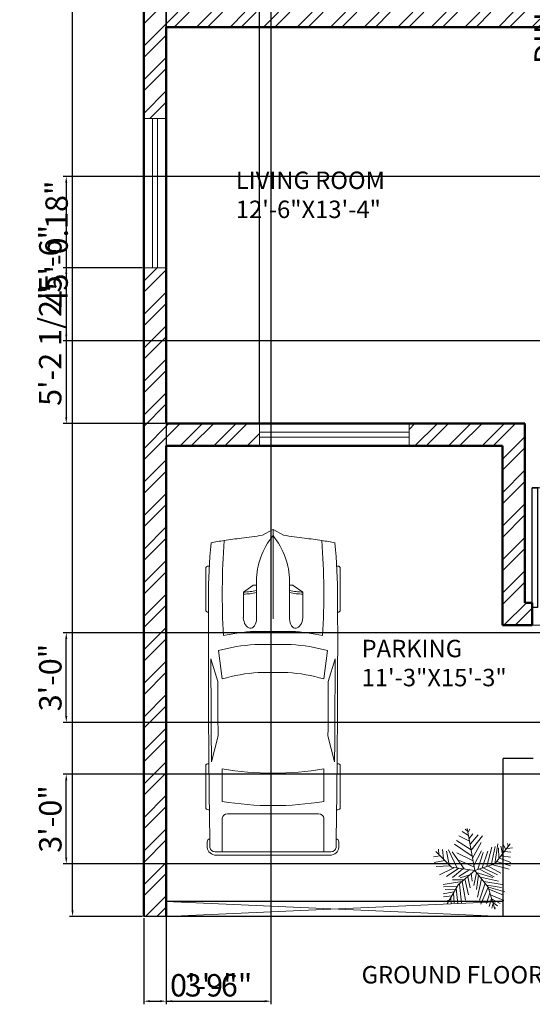
# Model space of a CAD drawing. Units: inches. Extents: x 1104 to 1745, y 678 to 1361.
# Tile 1 of 4: x 1181 to 1387, y 685 to 1080. Entities that reach past the tile are written whole.
import ezdxf

# ---------------------------------------------------------------- set-up
doc = ezdxf.new("R2010")
doc.units = ezdxf.units.IN
doc.linetypes.add('ACAD_ISO02W100', pattern=[15, 12, -3])
for name, color, linetype, lineweight in [('A-ANNO-DIMS', 2, 'Continuous', 18), ('A-ANNO-TEXT', 7, 'Continuous', 35), ('A-AREA-IDEN', 7, 'Continuous', 25), ('A-DOOR', 4, 'Continuous', 25), ('A-DOOR-HIDN', 4, 'ACAD_ISO02W100', 18), ('A-WALL', 7, 'Continuous', 50), ('A-WALL-PATT', 252, 'ACAD_ISO02W100', 13), ('C-PKNG-VEHI', 9, 'Continuous', 18), ('C-SITE', 8, 'Continuous', 25), ('L-PLNT', 94, 'Continuous', 18)]:
    doc.layers.add(name, color=color, linetype=linetype, lineweight=lineweight)
doc.layers.add('A-GLAZ', color=244, linetype='Continuous', lineweight=18, true_color=0x991b1e)
doc.layers.add('C-SITE-GATE', color=244, linetype='Continuous', lineweight=18, true_color=0x991b1e)
doc.styles.get("Standard").update_dxf_attribs({"font": 'arial.ttf'})
doc.dimstyles.new('ISO-25', dxfattribs={"dimtxt": 9, "dimasz": 2.5, "dimexe": 1.25, "dimexo": 0.625, "dimtad": 1, "dimlunit": 3, "dimtxsty": 'Standard', "dimcen": 2.5, "dimadec": 0, "dimazin": 0, "dimtfac": 1, "dimtmove": 0, "dimatfit": 3, "dimfxl": 1, "dimarcsym": 0})

# ---------------------------------------------------------------- blocks, each defined once
blk = doc.blocks.new('*U2')
for p, q in [((0, 0), (0, -6)), ((40, 0), (40, -6))]:
    blk.add_line(p, q)
blk.add_lwpolyline([(0, 0), (0, 40), (1.75, 40), (1.75, 0)], close=True)
blk.add_arc((0, 0), 40, 0, 90)
blk = doc.blocks.new('*D8')
at = {"layer": 'A-ANNO-DIMS', "color": 0, "lineweight": -2, "transparency": 16777216}
for p, q in [((1230.48, 1260.13), (1201.22, 1260.13)), ((1202.47, 722.45), (1202.47, 1257.63)), ((1230.48, 719.95), (1201.22, 719.95))]:
    blk.add_line(p, q, dxfattribs=at)
at = {"layer": 'A-ANNO-DIMS', "color": 0, "transparency": 16777216}
for points in [[(1202.05, 1257.63), (1202.88, 1257.63), (1202.47, 1260.13)], [(1202.05, 722.45), (1202.88, 722.45), (1202.47, 719.95)]]:
    blk.add_solid(points, dxfattribs=at)
at = {"layer": 'Defpoints', "color": 0, "transparency": 16777216}
for p in [(1202.47, 1260.13), (1231.11, 1260.13), (1231.11, 719.95)]:
    blk.add_point(p, dxfattribs=at)
at = {"layer": 'A-ANNO-DIMS', "color": 0, "transparency": 16777216, "insert": (1197.25, 990.04), "char_height": 9, "attachment_point": 5, "rotation": 90}
blk.add_mtext('45\'-0.18"', dxfattribs=at)
blk = doc.blocks.new('*U10')
for p, q in [((21.1, 37.41), (21.1, 36.83)), ((46.55, 38.89), (22.35, 38.89)), ((47.8, 37.39), (47.8, 37.41)), ((87.99, 31.87), (74.76, 35.92)), ((134.31, 35.6), (119.29, 31.78)), ((135.45, 37.07), (135.45, 37.41)), ((136.7, 38.89), (160.9, 38.89)), ((162.15, 37.41), (162.15, 36.77)), ((70.03, 31.54), (86.41, 29.35)), ((138.42, 29.35), (157.25, 29.35)), ((186.47, 29.35), (167.01, 29.35)), ((186.47, -33.5), (186.47, 33.5)), ((188.4, -32.76), (188.4, 32.76)), ((164.52, 26.39), (164.52, -26.39)), ((32.27, 11.63), (36.13, 17.17)), ((36.13, 17.17), (50.94, 17.17)), ((3.27, 6.13), (0.1, 0.41)), ((29.77, 9.51), (51.68, 9.51)), ((32.12, 9.51), (32.12, 11.15)), ((58.92, -10.77), (58.92, 10.77)), ((66.55, -10.53), (66.55, 10.53)), ((82.74, 8.5), (82.74, -8.5)), ((186.47, -10.53), (186.47, 10.53)), ((0, 0), (51.68, 0)), ((0.1, -0.41), (3.27, -6.13)), ((29.77, -9.51), (51.68, -9.51)), ((32.12, -9.51), (32.12, -11.15)), ((32.27, -11.63), (36.13, -17.17)), ((36.13, -17.17), (50.94, -17.17)), ((86.41, -29.35), (70.03, -31.54)), ((87.99, -31.87), (74.76, -35.92)), ((134.31, -35.6), (119.29, -31.78)), ((157.25, -29.35), (138.42, -29.35)), ((167.01, -29.35), (186.47, -29.35)), ((21.1, -37.41), (21.1, -36.83)), ((46.55, -38.89), (22.35, -38.89)), ((47.8, -37.39), (47.8, -37.41)), ((135.45, -37.07), (135.45, -37.41)), ((136.7, -38.89), (160.9, -38.89)), ((162.15, -37.41), (162.15, -36.77))]:
    blk.add_line(p, q)
for centre, major_axis, ratio, start_param, end_param in [((266.03, -27.52), (0, 313.31), 0.842304, 1.367076, 1.39176), ((41.19, -490.86), (0, 528.23), 0.842304, 0.00281, 0.075598), ((22.35, 37.41), (0, -1.48), 0.842304, 3.141593, 4.712389), ((64.48, -10555.62), (0, 10593.03), 0.842304, -0.013397, 0.002797), ((46.55, 37.41), (0, 1.48), 0.842304, -1.570796, 0), ((64.48, -10555.62), (0, -10591.55), 0.842304, 3.133765, 3.140441), ((136.7, 37.41), (0, -1.48), 0.842304, 3.141593, 4.712389), ((160.9, 37.41), (0, 1.48), 0.842304, -1.570796, 0), ((180.63, 35.84), (0, 2.22), 0.842304, -0.013017, 1.249894), ((64.48, -10556.36), (0, 10595.31), 0.842304, -0.013397, -0.013017), ((183.98, 33.5), (0, -2.96), 0.842304, 1.570796, 3.128196), ((183.98, 32.76), (0, -5.25), 0.842304, 1.570796, 3.128196), ((37.47, -593.96), (0, -623.33), 0.842304, 3.096046, 3.200911), ((134.4, 5.39), (0, -89.78), 0.842304, 4.449482, 4.652344), ((135.29, 5.39), (0, 81.77), 0.842304, 1.245306, 1.50788), ((149.6, 2.8), (0, -79.58), 0.842304, 4.372215, 4.640744), ((95.79, -3666.35), (0, -3698.24), 0.842304, 3.134049, 3.144098), ((17.08, 0), (0, 147.02), 0.842304, 4.511394, 4.913384), ((35.91, 0), (0, 147.02), 0.842304, 4.511394, 4.913384), ((167.01, 26.39), (0, 2.96), 0.842304, 0, 1.570796), ((259.18, -27.52), (0, -305.3), 0.842304, 4.528606, 4.561838), ((-204.49, 52.4), (0, -250.96), 0.842304, 1.385369, 1.434372), ((13.04, 17.01), (0, 27.42), 0.842304, 4.435146, 4.718221), ((14.2, 17.01), (0, 27.42), 0.842304, 4.435146, 4.718221), ((50.79, 13.34), (6.34, -0.36), 0.603834, -1.395552, 1.581315), ((32.75, 11.15), (0, 0.74), 0.842304, 0.879714, 1.570796), ((29.77, -46.66), (0, 56.17), 0.842304, 0, 0.590319), ((0.62, 0), (0, -0.74), 0.842304, 4.131459, 5.293319), ((29.77, 46.66), (0, 56.17), 0.842304, 2.551274, 3.141593), ((-204.49, -52.4), (0, 250.96), 0.842304, -1.434372, -1.385369), ((32.75, -11.15), (0, -0.74), 0.842304, 4.712389, 5.403472), ((13.04, -17.01), (0, -27.42), 0.842304, 1.564964, 1.848039), ((14.2, -17.01), (0, -27.42), 0.842304, 1.564964, 1.848039), ((134.4, -5.39), (0, -89.78), 0.842304, -1.510751, -1.307889), ((135.29, -5.39), (0, -81.77), 0.842304, -1.50788, -1.245306), ((149.6, -2.8), (0, -79.58), 0.842304, -1.499151, -1.230623), ((259.18, 27.52), (0, 305.3), 0.842304, 1.721348, 1.754579), ((266.03, 27.52), (0, 313.31), 0.842304, 1.749832, 1.774517), ((37.47, 593.96), (0, -623.33), 0.842304, -0.059319, 0.045547), ((167.01, -26.39), (0, -2.96), 0.842304, 4.712389, 6.283185), ((95.79, 3666.35), (0, -3698.24), 0.842304, -0.002505, 0.007544), ((183.98, -33.5), (0, 2.96), 0.842304, 3.15499, 4.712389), ((183.98, -32.76), (0, -5.25), 0.842304, 0.013397, 1.570796), ((41.19, 490.86), (0, -528.23), 0.842304, -0.075598, -0.00281), ((22.35, -37.41), (0, 1.48), 0.842304, 1.570796, 3.141593), ((64.48, 10555.62), (0, 10593.03), 0.842304, 3.138796, 3.15499), ((46.55, -37.41), (0, -1.48), 0.842304, 0, 1.570796), ((64.48, 10555.62), (0, -10591.55), 0.842304, 0.001152, 0.007828), ((136.7, -37.41), (0, -1.48), 0.842304, -1.570796, 0), ((160.9, -37.41), (0, 1.48), 0.842304, 3.141593, 4.712389), ((180.63, -35.84), (0, -2.22), 0.842304, -1.249894, 0.013017), ((64.48, 10556.36), (0, 10595.31), 0.842304, 3.15461, 3.15499)]:
    blk.add_ellipse(centre, major_axis=major_axis, ratio=ratio, start_param=start_param, end_param=end_param)
at = {"extrusion": (0, 0, -1)}
blk.add_ellipse((50.79, -13.34), major_axis=(6.34, 0.36), ratio=0.603834, start_param=-1.395552, end_param=1.581315, dxfattribs=at)
blk = doc.blocks.new('*U12')
for p, q in [((-10.186, 53.64), (-13.084, 55.962)), ((0, 0), (-10.5, 57)), ((-9.099, 51.782), (-6.563, 55.962)), ((-5.114, 28.097), (-24.676, 40.636)), ((-7.288, 39.707), (-21.778, 46.673)), ((-8.737, 47.138), (-17.069, 52.711)), ((-7.65, 43.423), (-2.578, 49.46)), ((-5.839, 35.992), (4.667, 48.067)), ((-5.114, 27.632), (10.463, 46.673)), ((-48.585, 21.131), (-49.309, 29.026)), ((-43.513, 28.561), (-42.427, 15.558)), ((-35.544, 28.097), (-24.314, 3.947)), ((-3.665, 19.273), (-27.574, 35.527)), ((-2.941, 16.486), (8.652, 37.85)), ((-1.129, 6.734), (9.014, 26.704)), ((16.259, 5.805), (23.142, 31.348)), ((22.055, 7.198), (27.489, 32.277)), ((27, 9), (48, 36)), ((27.127, 9.056), (31.112, 35.992)), ((31.836, 30.883), (32.561, 16.486)), ((35.096, 32.741), (37.27, 22.524)), ((38.719, 34.134), (41.979, 28.561)), ((43.791, 29.954), (51.036, 30.883)), ((44.153, 36.456), (45.239, 32.741)), ((-47.498, 19.737), (-55.83, 18.344)), ((-40.615, 13.7), (-55.105, 10.913)), ((-31.5, 4.5), (-52.5, 25.5)), ((-38.442, 26.239), (-34.819, 7.663)), ((-14.533, 2.09), (-30.834, 25.31)), ((-24.314, 23.917), (-2.941, 13.7)), ((-20.691, 13.7), (-1.129, 4.876)), ((3.942, 1.625), (11.187, 24.381)), ((10.101, 3.483), (17.708, 26.239)), ((33.285, 16.486), (48.862, 10.913)), ((36.183, 19.737), (48.137, 17.88)), ((40.53, 25.775), (48.862, 24.846)), ((-33.37, 6.269), (-52.207, 5.34)), ((-28.299, 3.483), (-47.86, -5.805)), ((-21.416, 3.018), (-38.079, -8.128)), ((0, 0), (-31.5, 4.5)), ((-15.982, 2.09), (-30.11, -9.521)), ((0, 0), (-22.5, -19.5)), ((-6.563, 1.161), (-21.416, -8.128)), ((0, 0), (27, 9)), ((0, 0), (18, -22.5)), ((6.478, 1.625), (26.04, -8.592)), ((11.187, 3.483), (30.749, -5.805)), ((18.07, 5.805), (35.096, -3.483)), ((24.229, 7.663), (46.688, 1.625)), ((29.662, 12.307), (48.137, 6.269)), ((-15.257, -12.772), (-30.11, -12.772)), ((-6.563, -5.805), (-19.967, -9.985)), ((-13.446, -11.378), (-8.737, -32.741)), ((-9.461, -8.592), (-6.201, -23.453)), ((-4.752, -3.483), (-3.665, -14.629)), ((2.493, -3.019), (-1.491, -20.202)), ((1.769, -2.555), (24.229, -9.521)), ((5.029, -6.27), (2.131, -25.775)), ((9.014, -11.378), (3.58, -35.992)), ((7.565, -9.056), (32.198, -14.629)), ((-17.431, -15.094), (-42.789, -18.809)), ((-24.314, -21.596), (-42.427, -22.06)), ((-26.849, -26.24), (-40.253, -25.775)), ((-22.5, -19.5), (-37.5, -45)), ((-25.038, -23.918), (-22.865, -45.281)), ((-20.691, -18.345), (-17.793, -44.352)), ((-17.069, -15.094), (-12.721, -40.172)), ((14.085, -16.951), (6.478, -40.172)), ((18.07, -22.524), (8.289, -45.745)), ((12.274, -15.094), (36.907, -18.809)), ((16.259, -19.738), (36.183, -22.989)), ((18, -22.5), (27, -52.5)), ((18.433, -22.524), (40.53, -29.026)), ((19.157, -25.311), (38.719, -33.206)), ((-28.299, -29.026), (-42.789, -31.348)), ((-30.834, -34.135), (-42.427, -35.528)), ((-34.457, -39.708), (-40.978, -42.494)), ((-32.646, -36.921), (-31.921, -44.352)), ((-29.023, -30.884), (-27.936, -43.887)), ((20.244, -30.419), (15.897, -44.816)), ((22.78, -37.85), (19.519, -48.532)), ((21.331, -32.741), (39.081, -40.636)), ((22.78, -38.314), (34.372, -44.816)), ((24.591, -45.745), (23.142, -50.854)), ((24.591, -43.423), (30.749, -47.603)), ((26.764, -49.925), (28.213, -50.854))]:
    blk.add_line(p, q)
blk = doc.blocks.new('WIN-GLASS-60IN')
for p, q in [((0, 2), (60, 2)), ((0, 0), (60, 0))]:
    blk.add_line(p, q)
blk = doc.blocks.new('*D31')
at = {"layer": 'A-ANNO-DIMS', "color": 0, "lineweight": -2, "transparency": 16777216}
for p, q in [((1398.91, 1057.87), (1398.91, 1160.54)), ((1411.93, 1057.87), (1397.66, 1057.87)), ((1398.91, 969.37), (1398.91, 1055.37)), ((1411.93, 966.87), (1397.66, 966.87))]:
    blk.add_line(p, q, dxfattribs=at)
at = {"layer": 'A-ANNO-DIMS', "color": 0, "transparency": 16777216}
for points in [[(1398.49, 1055.37), (1399.32, 1055.37), (1398.91, 1057.87)], [(1398.49, 969.37), (1399.32, 969.37), (1398.91, 966.87)]]:
    blk.add_solid(points, dxfattribs=at)
at = {"layer": 'Defpoints', "color": 0, "transparency": 16777216}
for p in [(1398.91, 1057.87), (1412.56, 1057.87), (1412.56, 966.87)]:
    blk.add_point(p, dxfattribs=at)
at = {"layer": 'A-ANNO-DIMS', "color": 0, "transparency": 16777216, "insert": (1393.63, 1110.45), "char_height": 9, "attachment_point": 5, "rotation": 90}
blk.add_mtext('DINING SET 7\'-7"', dxfattribs=at)
blk = doc.blocks.new('*D35')
at = {"layer": 'A-ANNO-DIMS', "color": 0, "lineweight": -2, "transparency": 16777216}
for p, q in [((1231.11, 719.32), (1231.11, 684.69)), ((1240.11, 719.32), (1240.11, 684.69)), ((1233.61, 685.94), (1237.61, 685.94)), ((1240.11, 685.94), (1267.78, 685.94))]:
    blk.add_line(p, q, dxfattribs=at)
at = {"layer": 'A-ANNO-DIMS', "color": 0, "transparency": 16777216}
for points in [[(1233.61, 686.36), (1233.61, 685.52), (1231.11, 685.94)], [(1237.61, 686.36), (1237.61, 685.52), (1240.11, 685.94)]]:
    blk.add_solid(points, dxfattribs=at)
at = {"layer": 'Defpoints', "color": 0, "transparency": 16777216}
for p in [(1231.11, 719.95), (1240.11, 719.95), (1240.11, 685.94)]:
    blk.add_point(p, dxfattribs=at)
at = {"layer": 'A-ANNO-DIMS', "color": 0, "transparency": 16777216, "insert": (1255.19, 691.16), "char_height": 9, "attachment_point": 5}
blk.add_mtext('0\'-9"', dxfattribs=at)
blk = doc.blocks.new('*D40')
at = {"layer": 'A-ANNO-DIMS', "color": 0, "lineweight": -2, "transparency": 16777216}
for p, q in [((1240.11, 1250.5), (1240.11, 684.69)), ((1282.11, 1250.5), (1282.11, 684.69)), ((1242.61, 685.94), (1279.61, 685.94))]:
    blk.add_line(p, q, dxfattribs=at)
at = {"layer": 'A-ANNO-DIMS', "color": 0, "transparency": 16777216}
for points in [[(1242.61, 686.36), (1242.61, 685.52), (1240.11, 685.94)], [(1279.61, 686.36), (1279.61, 685.52), (1282.11, 685.94)]]:
    blk.add_solid(points, dxfattribs=at)
at = {"layer": 'Defpoints', "color": 0, "transparency": 16777216}
for p in [(1240.11, 1251.13), (1282.11, 1251.13), (1282.11, 685.94)]:
    blk.add_point(p, dxfattribs=at)
at = {"layer": 'A-ANNO-DIMS', "color": 0, "transparency": 16777216, "insert": (1261.11, 691.16), "char_height": 9, "attachment_point": 5}
blk.add_mtext('3\'-6"', dxfattribs=at)
blk = doc.blocks.new('*D44')
at = {"layer": 'A-ANNO-DIMS', "color": 0, "lineweight": -2, "transparency": 16777216}
for p, q in [((1479.48, 1017.13), (1198.71, 1017.13)), ((1199.96, 1014.63), (1199.96, 953.63)), ((1479.48, 951.13), (1198.71, 951.13))]:
    blk.add_line(p, q, dxfattribs=at)
at = {"layer": 'A-ANNO-DIMS', "color": 0, "transparency": 16777216}
for points in [[(1199.54, 1014.63), (1200.37, 1014.63), (1199.96, 1017.13)], [(1199.54, 953.63), (1200.37, 953.63), (1199.96, 951.13)]]:
    blk.add_solid(points, dxfattribs=at)
at = {"layer": 'Defpoints', "color": 0, "transparency": 16777216}
for p in [(1480.11, 1017.13), (1199.96, 951.13), (1480.11, 951.13)]:
    blk.add_point(p, dxfattribs=at)
at = {"layer": 'A-ANNO-DIMS', "color": 0, "transparency": 16777216, "insert": (1194.74, 984.13), "char_height": 9, "attachment_point": 5, "rotation": 90}
blk.add_mtext('5\'-6"', dxfattribs=at)
blk = doc.blocks.new('*D47')
at = {"layer": 'A-ANNO-DIMS', "color": 0, "lineweight": -2, "transparency": 16777216}
for p, q in [((1479.48, 833.92), (1198.71, 833.92)), ((1199.96, 800.42), (1199.96, 831.42)), ((1479.48, 797.92), (1198.71, 797.92))]:
    blk.add_line(p, q, dxfattribs=at)
at = {"layer": 'A-ANNO-DIMS', "color": 0, "transparency": 16777216}
for points in [[(1199.54, 831.42), (1200.37, 831.42), (1199.96, 833.92)], [(1199.54, 800.42), (1200.37, 800.42), (1199.96, 797.92)]]:
    blk.add_solid(points, dxfattribs=at)
at = {"layer": 'Defpoints', "color": 0, "transparency": 16777216}
for p in [(1199.96, 833.92), (1480.11, 833.92), (1480.11, 797.92)]:
    blk.add_point(p, dxfattribs=at)
at = {"layer": 'A-ANNO-DIMS', "color": 0, "transparency": 16777216, "insert": (1194.73, 815.92), "char_height": 9, "attachment_point": 5, "rotation": 90}
blk.add_mtext('3\'-0"', dxfattribs=at)
blk = doc.blocks.new('*D52')
at = {"layer": 'A-ANNO-DIMS', "color": 0, "lineweight": -2, "transparency": 16777216}
for p, q in [((1230.48, 980.46), (1198.71, 980.46)), ((1199.96, 977.96), (1199.96, 920.42)), ((1239.48, 917.92), (1198.71, 917.92))]:
    blk.add_line(p, q, dxfattribs=at)
at = {"layer": 'A-ANNO-DIMS', "color": 0, "transparency": 16777216}
for points in [[(1199.54, 977.96), (1200.37, 977.96), (1199.96, 980.46)], [(1199.54, 920.42), (1200.37, 920.42), (1199.96, 917.92)]]:
    blk.add_solid(points, dxfattribs=at)
at = {"layer": 'Defpoints', "color": 0, "transparency": 16777216}
for p in [(1231.11, 980.46), (1199.96, 917.92), (1240.11, 917.92)]:
    blk.add_point(p, dxfattribs=at)
at = {"layer": 'A-ANNO-DIMS', "color": 0, "transparency": 16777216, "insert": (1194.68, 949.19), "char_height": 9, "attachment_point": 5, "rotation": 90}
blk.add_mtext('5\'-2 1/2"', dxfattribs=at)
blk = doc.blocks.new('*D54')
at = {"layer": 'A-ANNO-DIMS', "color": 0, "lineweight": -2, "transparency": 16777216}
for p, q in [((1485.48, 777.13), (1198.71, 777.13)), ((1199.96, 743.63), (1199.96, 774.63)), ((1485.48, 741.13), (1198.71, 741.13))]:
    blk.add_line(p, q, dxfattribs=at)
at = {"layer": 'A-ANNO-DIMS', "color": 0, "transparency": 16777216}
for points in [[(1199.54, 774.63), (1200.37, 774.63), (1199.96, 777.13)], [(1199.54, 743.63), (1200.37, 743.63), (1199.96, 741.13)]]:
    blk.add_solid(points, dxfattribs=at)
at = {"layer": 'Defpoints', "color": 0, "transparency": 16777216}
for p in [(1199.96, 777.13), (1486.11, 777.13), (1486.11, 741.13)]:
    blk.add_point(p, dxfattribs=at)
at = {"layer": 'A-ANNO-DIMS', "color": 0, "transparency": 16777216, "insert": (1194.73, 759.13), "char_height": 9, "attachment_point": 5, "rotation": 90}
blk.add_mtext('3\'-0"', dxfattribs=at)
blk = doc.blocks.new('*D56')
at = {"layer": 'A-ANNO-DIMS', "color": 0, "lineweight": -2, "transparency": 16777216}
for p, q in [((1240.11, 918.55), (1240.11, 1343.53)), ((1242.61, 1342.28), (1275.11, 1342.28)), ((1277.61, 918.55), (1277.61, 1343.53)), ((1277.61, 1342.28), (1326.25, 1342.28))]:
    blk.add_line(p, q, dxfattribs=at)
at = {"layer": 'A-ANNO-DIMS', "color": 0, "transparency": 16777216}
for points in [[(1242.61, 1342.7), (1242.61, 1341.86), (1240.11, 1342.28)], [(1275.11, 1342.7), (1275.11, 1341.86), (1277.61, 1342.28)]]:
    blk.add_solid(points, dxfattribs=at)
at = {"layer": 'Defpoints', "color": 0, "transparency": 16777216}
for p in [(1277.61, 1342.28), (1240.11, 917.92), (1277.61, 917.92)]:
    blk.add_point(p, dxfattribs=at)
at = {"layer": 'A-ANNO-DIMS', "color": 0, "transparency": 16777216, "insert": (1303.18, 1347.56), "char_height": 9, "attachment_point": 5}
blk.add_mtext('3\'-1 1/2"', dxfattribs=at)

msp = doc.modelspace()

# ---------------------------------------------------------------- hatches: boundary and pattern name
at = {"layer": 'A-WALL-PATT'}
h = msp.add_hatch(dxfattribs=at)
h.set_pattern_fill('ANSI32', color=256)
h.paths.add_polyline_path([(1277.606, 917.921), (1240.106, 917.921), (1240.106, 980.462), (1231.106, 980.462), (1231.106, 719.949), (1240.106, 719.949), (1240.106, 908.921), (1277.606, 908.921)])
h.paths.add_polyline_path([(1384.106, 917.921), (1337.606, 917.921), (1337.606, 908.921), (1375.106, 908.921), (1375.106, 836.921), (1387.106, 836.921), (1387.106, 844.121), (1387.106, 845.921), (1384.106, 845.921)])
h.paths.add_polyline_path([(1486.106, 849.129), (1543.106, 849.129), (1543.106, 855.129), (1540.106, 855.129), (1540.106, 951.129), (1612.106, 951.129), (1612.106, 941.864), (1621.106, 941.864), (1621.106, 986.665), (1612.106, 986.665), (1612.106, 957.129), (1486.106, 957.129), (1486.106, 1017.129), (1480.106, 1017.129), (1480.106, 951.129), (1534.106, 951.129), (1534.106, 855.129), (1480.106, 855.129), (1480.106, 845.921), (1476.166, 845.921), (1476.166, 836.921), (1480.106, 836.921), (1480.106, 833.921), (1486.106, 833.921)])
h.paths.add_polyline_path([(1441.89, 845.921), (1435.106, 845.921), (1435.106, 836.921), (1441.89, 836.921)])
h.paths.add_polyline_path([(1240.106, 1137.841), (1231.106, 1137.841), (1231.106, 1040.462), (1240.106, 1040.462), (1240.106, 1077.129), (1390.106, 1077.129), (1390.106, 1086.129), (1384.106, 1086.129), (1384.106, 1083.129), (1240.106, 1083.129)])
h.paths.add_polyline_path([(1621.106, 1146.091), (1612.106, 1146.091), (1612.106, 1083.129), (1468.106, 1083.129), (1468.106, 1086.129), (1462.106, 1086.129), (1462.106, 1077.129), (1480.106, 1077.129), (1612.106, 1077.129), (1612.106, 1046.665), (1621.106, 1046.665)])
h.paths.add_polyline_path([(1240.106, 1251.129), (1282.106, 1251.129), (1282.106, 1260.129), (1231.106, 1260.129), (1231.106, 1197.841), (1240.106, 1197.841)])
h.paths.add_polyline_path([(1418.05, 1260.129), (1342.106, 1260.129), (1342.106, 1251.129), (1384.106, 1251.129), (1384.106, 1122.129), (1390.106, 1122.129), (1390.106, 1149.129), (1429.106, 1149.129), (1429.106, 1155.129), (1390.106, 1155.129), (1390.106, 1251.129), (1418.05, 1251.129)])
h.paths.add_polyline_path([(1510.106, 1260.129), (1439.05, 1260.129), (1439.05, 1251.129), (1462.106, 1251.129), (1462.106, 1155.129), (1459.106, 1155.129), (1459.106, 1153.629), (1459.106, 1149.129), (1462.106, 1149.129), (1462.106, 1122.129), (1468.106, 1122.129), (1468.106, 1251.129), (1510.106, 1251.129)])
h.paths.add_polyline_path([(1621.106, 1260.129), (1570.106, 1260.129), (1570.106, 1251.129), (1612.106, 1251.129), (1612.106, 1206.091), (1621.106, 1206.091)])
h.paths.add_polyline_path([(1621.106, 920.864), (1612.106, 920.864), (1612.106, 855.129), (1573.106, 855.129), (1573.106, 849.129), (1612.106, 849.129), (1612.106, 809.56), (1621.106, 809.56)])
h.paths.add_polyline_path([(1621.106, 749.56), (1612.106, 749.56), (1612.106, 741.129), (1486.106, 741.129), (1486.106, 797.921), (1480.106, 797.921), (1480.106, 732.129), (1621.106, 732.129)])

# ---------------------------------------------------------------- linework, layer by layer
at = {"layer": 'A-DOOR-HIDN'}
msp.add_line((1387.106, 836.921), (1435.106, 836.921), dxfattribs=at)
at = {"layer": 'A-GLAZ'}
for points in [[(1240.106, 1040.462), (1240.106, 980.462), (1231.106, 980.462), (1231.106, 1040.462)], [(1277.606, 917.921), (1337.606, 917.921), (1337.606, 908.921), (1277.606, 908.921)]]:
    msp.add_lwpolyline(points, close=True, dxfattribs=at)
at = {"layer": 'A-WALL'}
for p, q in [((1231.106, 1260.129), (1231.106, 719.949)), ((1240.106, 1077.129), (1390.106, 1077.129)), ((1240.106, 1077.129), (1240.106, 917.921)), ((1240.106, 917.921), (1384.106, 917.921)), ((1384.106, 917.921), (1384.106, 845.921)), ((1240.106, 908.921), (1375.106, 908.921)), ((1240.106, 908.921), (1240.106, 719.949)), ((1375.106, 908.921), (1375.106, 836.921)), ((1384.106, 845.921), (1387.106, 845.921)), ((1387.106, 845.921), (1387.106, 836.921)), ((1375.106, 836.921), (1387.106, 836.921))]:
    msp.add_line(p, q, dxfattribs=at)
at = {"layer": 'C-SITE'}
for p, q in [((1375.451, 719.949), (1375.451, 783.475)), ((1387.451, 783.475), (1375.451, 783.475)), ((1375.451, 725.949), (1240.106, 725.949)), ((1480.106, 719.949), (1231.106, 719.949))]:
    msp.add_line(p, q, dxfattribs=at)
at = {"layer": 'C-SITE-GATE'}
for p, q in [((1240.106, 719.949), (1375.451, 725.949)), ((1375.451, 719.949), (1240.106, 725.949))]:
    msp.add_line(p, q, dxfattribs=at)

# ---------------------------------------------------------------- block references
at = {"layer": 'A-DOOR', "xscale": 1.200000000000001, "yscale": 1.200000000000001, "zscale": 1.200000000000001}
msp.add_blockref('*U2', (1387.106, 844.121), dxfattribs=at)
at = {"layer": 'A-GLAZ', "rotation": 90}
msp.add_blockref('WIN-GLASS-60IN', (1236.606, 980.462), dxfattribs=at)
at = {"layer": 'A-GLAZ'}
msp.add_blockref('WIN-GLASS-60IN', (1277.606, 912.421), dxfattribs=at)
at = {"layer": 'C-PKNG-VEHI', "xscale": 0.694103067062351, "yscale": 0.694103067062351, "zscale": 0.694103067062351, "rotation": 270}
msp.add_blockref('*U10', (1282.982, 875.349), dxfattribs=at)
at = {"layer": 'L-PLNT', "xscale": 0.2968663969365763, "yscale": 0.2968663969365763, "zscale": 0.2968663969365763}
msp.add_blockref('*U12', (1364.018, 738.432), dxfattribs=at)

# ---------------------------------------------------------------- texts
at = {"layer": 'A-ANNO-TEXT', "insert": (1318.552, 700.062), "char_height": 7, "attachment_point": 1}
msp.add_mtext_dynamic_manual_height_columns('GROUND FLOOR PLAN', width=110.84972, gutter_width=12.5, heights=[0], dxfattribs=at)
at = {"layer": 'A-AREA-IDEN', "char_height": 7, "attachment_point": 1}
for s, width, insert in [('LIVING ROOM\\P12\'-6"X13\'-4"', 66.12074, (1268.038, 1019.131)), ('PARKING\\P11\'-3"X15\'-3"', 55.15613, (1318.552, 831.08))]:
    msp.add_mtext_dynamic_manual_height_columns(s, width=width, gutter_width=12.5, heights=[0], dxfattribs=dict(at, insert=insert))

# ---------------------------------------------------------------- dimensions: what is measured, and where the dimension line sits
at = {"layer": 'A-ANNO-DIMS'}
for base, p1, p2, picture, middle in [((1277.606, 1342.279), (1240.106, 917.921), (1277.606, 917.921), '*D56', (1303.176, 1347.56)), ((1282.106, 685.941), (1240.106, 1251.129), (1282.106, 1251.129), '*D40', (1261.106, 691.164)), ((1240.106, 685.941), (1231.106, 719.949), (1240.106, 719.949), '*D35', (1255.194, 691.161))]:
    dim = msp.add_linear_dim(base=base, p1=p1, p2=p2, dimstyle='ISO-25', override={"dimdec": 1, "dimlfac": 1, "dimrnd": 0, "dimzin": 1, "dimdsep": 46, "dimlunit": 4, "dimfrac": 2}, dxfattribs=at)
    dim.commit()
    dim.dimension.update_dxf_attribs({"geometry": picture, "text_midpoint": middle})
for base, p1, p2, override, picture, middle in [((1202.467, 1260.129), (1231.106, 719.949), (1231.106, 1260.129), {"dimclrd": 0, "dimclre": 0, "dimclrt": 0}, '*D8', (1197.247, 990.039)), ((1199.956, 951.129), (1480.106, 1017.129), (1480.106, 951.129), {"dimdec": 1, "dimlfac": 1, "dimrnd": 0, "dimzin": 1, "dimdsep": 46, "dimlunit": 4, "dimfrac": 2}, '*D44', (1194.736, 984.129)), ((1199.956, 917.921), (1231.106, 980.462), (1240.106, 917.921), {"dimdec": 1, "dimlfac": 1, "dimrnd": 0, "dimzin": 1, "dimdsep": 46, "dimlunit": 4, "dimfrac": 2}, '*D52', (1194.678, 949.191)), ((1199.956, 833.921), (1480.106, 797.921), (1480.106, 833.921), {"dimdec": 1, "dimlfac": 1, "dimrnd": 0, "dimzin": 1, "dimdsep": 46, "dimlunit": 4, "dimfrac": 2}, '*D47', (1194.733, 815.921)), ((1199.956, 777.129), (1486.106, 741.129), (1486.106, 777.129), {"dimdec": 1, "dimlfac": 1, "dimrnd": 0, "dimzin": 1, "dimdsep": 46, "dimlunit": 4, "dimfrac": 2}, '*D54', (1194.733, 759.129))]:
    dim = msp.add_linear_dim(base=base, p1=p1, p2=p2, angle=90, dimstyle='ISO-25', override=override, dxfattribs=at)
    dim.commit()
    dim.dimension.update_dxf_attribs({"geometry": picture, "text_midpoint": middle})
dim = msp.add_linear_dim(base=(1398.906, 1057.865), p1=(1412.556, 966.865), p2=(1412.556, 1057.865), angle=90, text='DINING SET <>', dimstyle='ISO-25', override={"dimdec": 1, "dimlfac": 1, "dimrnd": 0, "dimzin": 1, "dimdsep": 46, "dimlunit": 4, "dimfrac": 2}, dxfattribs=at)
dim.commit()
dim.dimension.update_dxf_attribs({"geometry": '*D31', "text_midpoint": (1393.627, 1110.45)})

doc.saveas('drawing.dxf')
